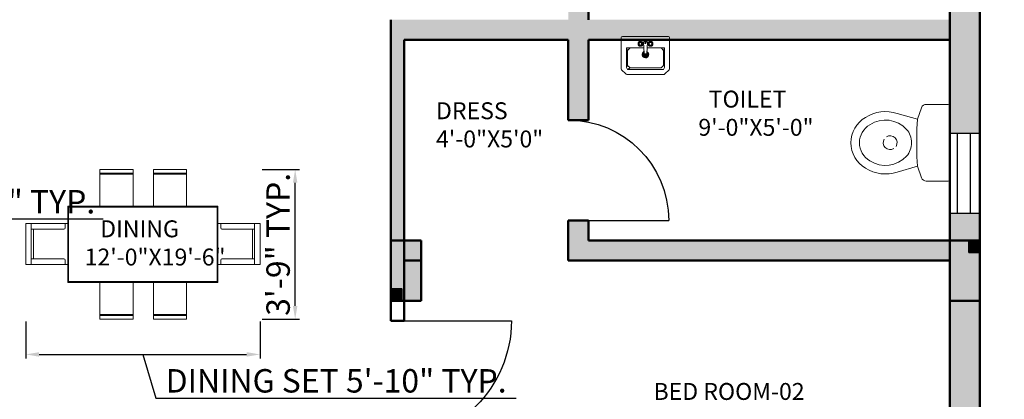
# Model space of a CAD drawing. Units: inches. Extents: x -7 to 1228, y -146 to 1091.
# Tile 23 of 88: x 269 to 563, y 194 to 307. Entities that reach past the tile are written whole.
import ezdxf

# ---------------------------------------------------------------- set-up
doc = ezdxf.new("R2010")
doc.units = ezdxf.units.IN
for name, color, linetype, lineweight in [('A-ANNO-DIMS', 2, 'Continuous', 18), ('A-AREA-IDEN', 7, 'Continuous', 18), ('A-COLS', 6, 'Continuous', 35), ('A-DOOR', 4, 'Continuous', 25), ('A-FLOR-FIXT', 8, 'Continuous', 18), ('A-FURN', 8, 'Continuous', 18), ('A-GLAZ', 175, 'Continuous', 25), ('A-WALL', 7, 'Continuous', 50), ('A-WALL-PATT', 251, 'Continuous', 13)]:
    doc.layers.add(name, color=color, linetype=linetype, lineweight=lineweight)
doc.styles.get("Standard").update_dxf_attribs({"font": 'arial.ttf'})
doc.dimstyles.new('ISO-25', dxfattribs={"dimtxt": 7, "dimasz": 4, "dimexe": 1.25, "dimexo": 0.625, "dimtad": 1, "dimdec": 1, "dimlunit": 3, "dimtxsty": 'Standard', "dimcen": 2.5, "dimadec": 0, "dimazin": 0, "dimtfac": 1, "dimtdec": 1, "dimtmove": 1, "dimatfit": 3, "dimfxl": 1, "dimarcsym": 0})

# ---------------------------------------------------------------- blocks, each defined once
blk = doc.blocks.new('A$C7B5C7CD4')
at = {"ltscale": 20}
for p, q in [((0.243, 0.625), (0.011, 0.625)), ((0.243, 0.625), (0.475, 0.625)), ((0, 0.614), (0, 0.4765)), ((0.486, 0.614), (0.486, 0.4765)), ((0.0212, 0.4467), (0.0946, 0.4214)), ((0.4648, 0.4467), (0.3914, 0.4214)), ((0.0946, 0.4214), (0.0576, 0.293)), ((0.0946, 0.4214), (0.1544, 0.4173)), ((0.3316, 0.4173), (0.1544, 0.4173)), ((0.3914, 0.4214), (0.3316, 0.4173)), ((0.3914, 0.4214), (0.4284, 0.293))]:
    blk.add_line(p, q, dxfattribs=at)
for centre, radius, start, end in [((0.011, 0.614), 0.011, 90, 180), ((0.475, 0.614), 0.011, 0, 90), ((0.0315, 0.4765), 0.0315, 180, 251), ((0.4545, 0.4765), 0.0315, 289, 0), ((0.24, 0.2602), 0.123, 88.61575, 131.74141), ((0.246, 0.2602), 0.123, 48.25859, 91.38425), ((0.2796, 0.219), 0.18, 132.42075, 213.28898), ((0.2064, 0.219), 0.18, 326.71102, 47.57925), ((0.2796, 0.219), 0.234, 161.58462, 212.87535), ((0.2064, 0.219), 0.234, 327.12465, 18.41538), ((0.243, 0.185), 0.185, 210.1745, 270), ((0.243, 0.185), 0.131, 209.62919, 270), ((0.243, 0.185), 0.131, 270, 330.37081), ((0.243, 0.185), 0.185, 270, 329.8255)]:
    blk.add_arc(centre, radius, start, end, dxfattribs=at)
for start, end in [(58.17854, 211.82146), (238.17854, 31.82146)]:
    blk.add_arc((0.2426, 0.2481), 0.0439, start, end)
blk = doc.blocks.new('A$C317A697B')
for p, q in [((-116, 441), (-514, 441)), ((-514, 441), (-514, 0)), ((-116, 398), (-514, 398)), ((-116, 385), (-514, 385)), ((-116, 0), (-116, 441)), ((523, 441), (125, 441)), ((125, 441), (125, 0)), ((523, 398), (125, 398)), ((523, 385), (125, 385)), ((523, 0), (523, 441)), ((-899, -912), (-899, 0)), ((-899, 0), (899, 0)), ((899, 0), (899, -912)), ((-889, -902), (-889, -10)), ((-889, -10), (889, -10)), ((889, -10), (889, -902)), ((-899, -205), (-1402, -205)), ((-1402, -205), (-1402, -699)), ((-1336, -205), (-1336, -699)), ((-932, -205), (-932, -259)), ((899, -205), (1402, -205)), ((932, -205), (932, -259)), ((1336, -205), (1336, -699)), ((1402, -205), (1402, -699)), ((-946, -274), (-1336, -274)), ((-1311, -274), (-1311, -630)), ((946, -274), (1336, -274)), ((1311, -274), (1311, -630)), ((-1402, -699), (-899, -699)), ((-946, -630), (-1336, -630)), ((-932, -699), (-932, -645)), ((1402, -699), (899, -699)), ((932, -699), (932, -645)), ((946, -630), (1336, -630)), ((899, -912), (-899, -912)), ((889, -902), (-889, -902)), ((-514, -1353), (-514, -912)), ((-116, -912), (-116, -1353)), ((125, -1353), (125, -912)), ((523, -912), (523, -1353)), ((-116, -1297), (-514, -1297)), ((-116, -1309), (-514, -1309)), ((-116, -1353), (-514, -1353)), ((523, -1297), (125, -1297)), ((523, -1309), (125, -1309)), ((523, -1353), (125, -1353))]:
    blk.add_line(p, q)
for centre, start, end in [((-946, -259), 270, 0), ((946, -259), 180, 270), ((-946, -645), 0, 90), ((946, -645), 90, 180)]:
    blk.add_arc(centre, 14.7, start, end)
blk = doc.blocks.new('A$C4CB854FF')
for p, q in [((0, 0.3675), (0, 0.0552)), ((0.4725, 0.38), (0.0125, 0.38)), ((0.1677, 0.2932), (0.1677, 0.318)), ((0.1745, 0.2919), (0.1745, 0.3194)), ((0.1773, 0.3221), (0.2048, 0.3221)), ((0.1787, 0.329), (0.2034, 0.329)), ((0.2075, 0.3194), (0.2075, 0.2919)), ((0.2144, 0.318), (0.2144, 0.2932)), ((0.2279, 0.2104), (0.2213, 0.3235)), ((0.2337, 0.329), (0.2502, 0.329)), ((0.2625, 0.3235), (0.256, 0.2104)), ((0.2694, 0.318), (0.2694, 0.2932)), ((0.2763, 0.3194), (0.2763, 0.2919)), ((0.3065, 0.3221), (0.279, 0.3221)), ((0.3052, 0.329), (0.2804, 0.329)), ((0.3093, 0.2919), (0.3093, 0.3194)), ((0.3162, 0.2932), (0.3162, 0.318)), ((0.485, 0.0552), (0.485, 0.3675)), ((0.05, 0.265), (0.2247, 0.265)), ((0.06, 0.24), (0.05, 0.265)), ((0.05, 0.07), (0.05, 0.265)), ((0.085, 0.265), (0.06, 0.24)), ((0.06, 0.24), (0.06, 0.09)), ((0.2048, 0.2891), (0.1773, 0.2891)), ((0.2034, 0.2822), (0.1787, 0.2822)), ((0.2152, 0.1984), (0.2694, 0.1984)), ((0.2297, 0.2066), (0.2165, 0.2066)), ((0.2272, 0.2149), (0.2208, 0.2149)), ((0.2505, 0.2052), (0.2334, 0.2052)), ((0.2681, 0.2066), (0.2541, 0.2066)), ((0.2638, 0.2149), (0.2566, 0.2149)), ((0.2591, 0.265), (0.43, 0.265)), ((0.279, 0.2891), (0.3065, 0.2891)), ((0.2804, 0.2822), (0.3052, 0.2822)), ((0.395, 0.265), (0.42, 0.24)), ((0.42, 0.24), (0.43, 0.265)), ((0.42, 0.24), (0.42, 0.09)), ((0.43, 0.07), (0.43, 0.265)), ((0.2681, 0.1901), (0.2165, 0.1901)), ((0.2638, 0.1819), (0.2208, 0.1819)), ((0.2533, 0.1736), (0.2313, 0.1736)), ((0.0037, 0.0463), (0.0463, 0.0037)), ((0.05, 0.07), (0.06, 0.05)), ((0.06, 0.09), (0.085, 0.065)), ((0.42, 0.05), (0.06, 0.05)), ((0.085, 0.065), (0.395, 0.065)), ((0.42, 0.09), (0.395, 0.065)), ((0.395, 0.065), (0.42, 0.05)), ((0.42, 0.09), (0.43, 0.07)), ((0.43, 0.07), (0.42, 0.05)), ((0.4387, 0.0037), (0.4813, 0.0463)), ((0.0552, 0), (0.4298, 0))]:
    blk.add_line(p, q)
for centre, radius in [((0.191, 0.3056), 0.0165), ((0.191, 0.3056), 0.0127), ((0.2419, 0.3152), 0.00688), ((0.2419, 0.3152), 0.00344), ((0.2928, 0.3056), 0.0165), ((0.2928, 0.3056), 0.0127)]:
    blk.add_circle(centre, radius)
for centre, radius, start, end in [((0.0125, 0.3675), 0.0125, 90, 180), ((0.1787, 0.318), 0.011, 90, 180), ((0.1773, 0.3194), 0.00275, 90, 180), ((0.2034, 0.318), 0.011, 0, 90), ((0.2048, 0.3194), 0.00275, 360, 90), ((0.2329, 0.314), 0.015, 87.19754, 140.72744), ((0.2509, 0.314), 0.015, 39.27256, 92.80246), ((0.2804, 0.318), 0.011, 90, 180), ((0.279, 0.3194), 0.00275, 90, 180), ((0.3052, 0.318), 0.011, 0, 90), ((0.3065, 0.3194), 0.00275, 360, 90), ((0.4725, 0.3675), 0.0125, 0, 90), ((0.1787, 0.2932), 0.011, 180, 270), ((0.1773, 0.2919), 0.00275, 180, 270), ((0.2034, 0.2932), 0.011, 270, 0), ((0.2048, 0.2919), 0.00275, 270, 0), ((0.2423, 0.1984), 0.033, 118.68833, 62.86857), ((0.2423, 0.1984), 0.0271, 124.77581, 57.22467), ((0.2334, 0.2107), 0.0055, 183.3274, 270), ((0.2505, 0.2107), 0.0055, 270, 356.6726), ((0.2804, 0.2932), 0.011, 180, 270), ((0.279, 0.2919), 0.00275, 180, 270), ((0.3052, 0.2932), 0.011, 270, 360), ((0.3065, 0.2919), 0.00275, 270, 0), ((0.0125, 0.0552), 0.0125, 180, 225), ((0.0552, 0.0125), 0.0125, 225, 270), ((0.4298, 0.0125), 0.0125, 270, 315), ((0.4725, 0.0552), 0.0125, 315, 0)]:
    blk.add_arc(centre, radius, start, end)
blk = doc.blocks.new('WIN-24')
for p, q in [((0, 0), (0, 24)), ((0, 24), (9, 24)), ((2.34, 0), (2.34, 24)), ((2.34, 24), (6.14, 24)), ((6.14, 24), (6.14, 0)), ((9, 24), (9, 0)), ((9, 0), (0, 0))]:
    blk.add_line(p, q)
blk = doc.blocks.new('DOOR-750')
blk.add_line((30, 30), (30, 0))
blk.add_arc((30, 30), 30, 180, 270)
blk = doc.blocks.new('DOOR-900')
blk.add_line((36, 0), (36, 36))
blk.add_arc((36, 0), 36, 90, 180)
blk = doc.blocks.new('*D32')
at = {"layer": 'A-ANNO-DIMS', "color": 0, "lineweight": -2, "transparency": 16777216}
for p, q in [((159.65, 262.03), (159.65, 259.24)), ((174.13, 262.03), (174.13, 259.24)), ((170.13, 260.49), (163.65, 260.49)), ((166.89, 260.49), (170.8, 247.44)), ((170.8, 247.44), (294.04, 247.44))]:
    blk.add_line(p, q, dxfattribs=at)
at = {"layer": 'A-ANNO-DIMS', "color": 0, "transparency": 16777216}
for points in [[(163.65, 261.15), (163.65, 259.82), (159.65, 260.49)], [(170.13, 261.15), (170.13, 259.82), (174.13, 260.49)]]:
    blk.add_solid(points, dxfattribs=at)
at = {"layer": 'Defpoints', "color": 0, "transparency": 16777216}
for p in [(159.65, 262.66), (174.13, 262.66), (159.65, 260.49)]:
    blk.add_point(p, dxfattribs=at)
at = {"layer": 'A-ANNO-DIMS', "color": 0, "transparency": 16777216, "insert": (232.42, 251.68), "char_height": 7, "attachment_point": 5}
blk.add_mtext('SINK / BASIN 1\'-2 1/2" TYP.', dxfattribs=at)
blk = doc.blocks.new('*D36')
at = {"layer": 'A-ANNO-DIMS', "color": 0, "lineweight": -2, "transparency": 16777216}
for p, q in [((270.86, 216.83), (270.86, 205.7)), ((340.87, 216.83), (340.87, 205.7)), ((274.86, 206.95), (336.87, 206.95)), ((305.87, 206.95), (309.78, 193.91)), ((309.78, 193.91), (417.47, 193.91))]:
    blk.add_line(p, q, dxfattribs=at)
at = {"layer": 'A-ANNO-DIMS', "color": 0, "transparency": 16777216}
for points in [[(274.86, 207.62), (274.86, 206.28), (270.86, 206.95)], [(336.87, 207.62), (336.87, 206.28), (340.87, 206.95)]]:
    blk.add_solid(points, dxfattribs=at)
at = {"layer": 'Defpoints', "color": 0, "transparency": 16777216}
for p in [(270.86, 217.45), (340.87, 217.45), (340.87, 206.95)]:
    blk.add_point(p, dxfattribs=at)
at = {"layer": 'A-ANNO-DIMS', "color": 0, "transparency": 16777216, "insert": (363.62, 198.15), "char_height": 7, "attachment_point": 5}
blk.add_mtext('DINING SET 5\'-10" TYP.', dxfattribs=at)
blk = doc.blocks.new('*D37')
at = {"layer": 'A-ANNO-DIMS', "color": 0, "lineweight": -2, "transparency": 16777216}
for p, q in [((341.5, 262.25), (352.63, 262.25)), ((351.38, 221.45), (351.38, 258.25)), ((341.5, 217.45), (352.63, 217.45))]:
    blk.add_line(p, q, dxfattribs=at)
at = {"layer": 'A-ANNO-DIMS', "color": 0, "transparency": 16777216}
for points in [[(350.71, 258.25), (352.04, 258.25), (351.38, 262.25)], [(350.71, 221.45), (352.04, 221.45), (351.38, 217.45)]]:
    blk.add_solid(points, dxfattribs=at)
at = {"layer": 'Defpoints', "color": 0, "transparency": 16777216}
for p in [(340.87, 262.25), (351.38, 262.25), (340.87, 217.45)]:
    blk.add_point(p, dxfattribs=at)
at = {"layer": 'A-ANNO-DIMS', "color": 0, "transparency": 16777216, "insert": (347.18, 239.85), "char_height": 7, "attachment_point": 5, "rotation": 90}
blk.add_mtext('3\'-9" TYP.', dxfattribs=at)

msp = doc.modelspace()

# ---------------------------------------------------------------- hatches: boundary and pattern name
at = {"layer": 'A-COLS'}
h = msp.add_hatch(color=256, dxfattribs=at)
h.dxf.hatch_style = 1
h.paths.add_polyline_path([(380, 226.55), (383.29, 226.55), (383.29, 223), (389, 223), (389, 241), (380, 241)])
h = msp.add_hatch(color=256, dxfattribs=at)
h.dxf.hatch_style = 1
h.paths.add_polyline_path([(556, 237.45), (552.71, 237.45), (552.71, 241), (547, 241), (547, 223), (556, 223)])
h = msp.add_hatch(color=256, dxfattribs=at)
h.dxf.hatch_style = 1
h.paths.add_polyline_path([(556, 237.45), (556, 241), (552.71, 241), (552.71, 237.45)])
h = msp.add_hatch(color=256, dxfattribs=at)
h.dxf.hatch_style = 1
h.paths.add_polyline_path([(380, 226.55), (380, 223), (383.29, 223), (383.29, 226.55)])
at = {"layer": 'A-WALL-PATT'}
h = msp.add_hatch(color=256, dxfattribs=at)
h.dxf.hatch_style = 1
h.paths.add_polyline_path([(69, 568), (60, 568), (60, 493), (63.29, 493), (69, 493)])
h.paths.add_polyline_path([(69, 662.41), (60, 662.41), (60, 586), (69, 586)], flags=17)
h.paths.add_polyline_path([(69, 723), (184, 723), (184, 734), (179, 734), (179, 728), (69, 728), (69, 741.62), (60, 741.62), (60, 698.41), (69, 698.41)], flags=17)
h.paths.add_polyline_path([(69, 782), (231, 782), (231, 728), (231, 723), (231, 586), (236, 586), (236, 787), (69, 787), (69, 800.13), (60, 800.13), (60, 765.62), (69, 765.62)])
h.paths.add_polyline_path([(184, 842), (189, 842), (189, 848), (173, 848), (173, 842), (179, 842), (179, 787), (184, 787)])
h.paths.add_polyline_path([(118.22, 69), (69, 69), (69, 60), (118.22, 60)])
h.paths.add_polyline_path([(227, 69), (154.22, 69), (154.22, 60), (227, 60)])
h.paths.add_polyline_path([(236, 60), (232.71, 60), (227, 60), (227, 36), (236, 36)])
h.paths.add_polyline_path([(389, 60), (380, 60), (380, 36), (389, 36)])
h.paths.add_polyline_path([(384, 181), (380, 181), (380, 115), (380, 78), (384, 78)])
h.paths.add_polyline_path([(380, 115), (334.55, 115), (334.55, 109), (380, 109)])
h.paths.add_polyline_path([(274.55, 115), (236, 115), (236, 201), (232.71, 201), (231, 201), (231, 78), (236, 78), (236, 109), (274.55, 109)])
h.paths.add_polyline_path([(69, 123), (60, 123), (60, 78), (69, 78)])
h.paths.add_polyline_path([(69, 201), (60, 201), (60, 159), (69, 159)])
h.paths.add_polyline_path([(143, 219), (69, 219), (69, 213), (143, 213)], flags=17)
h.paths.add_polyline_path([(189, 219), (184, 219), (184, 274), (231, 274), (231, 219), (236, 219), (236, 279), (184, 279), (184, 297), (179, 297), (179, 279), (69, 279), (69, 290.91), (60, 290.91), (60, 262.18), (69, 262.18), (69, 274), (179, 274), (179, 219), (173, 219), (173, 213), (189, 213)])
h.paths.add_polyline_path([(69, 238.18), (60, 238.18), (60, 219), (69, 219)], flags=17)
h.paths.add_polyline_path([(69, 333), (60, 333), (60, 314.91), (69, 314.91), (69, 316.96)])
h.paths.add_polyline_path([(190, 338), (184, 338), (69, 338), (69, 333), (179, 333), (179, 327), (184, 327), (184, 333.02), (190, 333.05)])
h.paths.add_polyline_path([(69, 386.81), (60, 386.81), (60, 351), (69, 351)])
h.paths.add_polyline_path([(69, 475), (60, 475), (60, 422.81), (69, 422.81)])
h.paths.add_polyline_path([(236, 475), (231, 475), (231, 351.24), (236, 351.24)])
h.paths.add_polyline_path([(384, 475), (380, 475), (380, 362), (384, 362)])
h.paths.add_polyline_path([(547, 307), (439, 307), (439, 356), (445, 356), (445, 362), (433, 362), (433, 307), (380, 307), (380, 244), (380, 241), (384, 241), (384, 301), (433, 301), (433, 277), (439, 277), (439, 301), (547, 301)])
h.paths.add_polyline_path([(547, 241), (439, 241), (439, 247), (433, 247), (433, 235), (547, 235)])
h.paths.add_polyline_path([(450, 69), (440.29, 69), (424.89, 69), (389, 69), (389, 60), (450, 60)])
h.paths.add_polyline_path([(547, 69), (486, 69), (486, 60), (547, 60)])
h.paths.add_polyline_path([(556, 148.27), (547, 148.27), (547, 78), (556, 78)])
h.paths.add_polyline_path([(556, 223), (547, 223), (547, 195), (547, 184.27), (556, 184.27)])
h.paths.add_polyline_path([(556, 311.19), (547, 311.19), (547, 273.08), (556, 273.08)])
h.paths.add_polyline_path([(556, 344), (552.71, 344), (547, 344), (547, 335.19), (556, 335.19)])
h.paths.add_polyline_path([(556, 249.08), (547, 249.08), (547, 241), (556, 241)])
h.paths.add_polyline_path([(547, 362), (475, 362), (475, 356), (547, 356)], flags=0)
h.paths.add_polyline_path([(556, 399.62), (547, 399.62), (547, 362), (556, 362)])
h.paths.add_polyline_path([(556, 475), (547, 475), (547, 435.62), (556, 435.62)])
h.paths.add_polyline_path([(547, 493), (389, 493), (389, 487), (547, 487)])
h.paths.add_polyline_path([(380, 493), (278, 493), (278, 487), (380, 487)])
h.paths.add_polyline_path([(227, 493), (69, 493), (69, 487), (227, 487)])
h.paths.add_polyline_path([(643, 122.44), (634, 122.44), (634, 78), (643, 78)])
h.paths.add_polyline_path([(702.5, 69), (692.79, 69), (677.39, 69), (643, 69), (643, 60), (702.5, 60)])
h.paths.add_polyline_path([(798, 69), (738.5, 69), (738.5, 60), (798, 60)])
h.paths.add_polyline_path([(807, 60), (803.71, 60), (798, 60), (798, 36), (807, 36)])
h.paths.add_polyline_path([(807, 109), (846.75, 109), (846.75, 115), (807, 115), (807, 159), (802, 159), (802, 78), (807, 78)])
h.paths.add_polyline_path([(807, 201), (802, 201), (802, 195), (807, 195)])
h.paths.add_polyline_path([(643, 201), (634, 201), (634, 158.44), (643, 158.44)])
h.paths.add_polyline_path([(756, 225), (751, 225), (751, 219), (643, 219), (643, 213), (756, 213)])
h.paths.add_polyline_path([(643, 240.85), (634, 240.85), (634, 219), (643, 219)])
h.paths.add_polyline_path([(643, 274), (643, 288.63), (634, 288.63), (634, 264.85), (643, 264.85)])
h.paths.add_polyline_path([(802, 279), (756, 279), (756, 297), (751, 297), (751, 279), (643, 279), (643, 274), (751, 274), (751, 255), (756, 255), (756, 274), (802, 274)])
h.paths.add_polyline_path([(807, 333), (803.71, 333), (802, 333), (802, 279), (802, 274), (802, 219), (807, 219)])
h.paths.add_polyline_path([(956, 182), (951, 182), (951, 115), (906.75, 115), (906.75, 109), (951, 109), (951, 78), (956, 78)])
h.paths.add_polyline_path([(960, 60), (951, 60), (951, 36), (960, 36)])
h.paths.add_polyline_path([(1021, 69), (1005.78, 69), (960, 69), (960, 60), (1021, 60)])
h.paths.add_polyline_path([(956, 224), (951, 224), (951, 218), (956, 218)])
h.paths.add_polyline_path([(956, 302), (1004, 302), (1004, 278), (1010, 278), (1010, 302), (1118, 302), (1118, 290.81), (1127, 290.81), (1127, 326.97), (1118, 326.97), (1118, 320.97), (1118, 307), (1010, 307), (1010, 356), (1016, 356), (1016, 362), (1004, 362), (1004, 307), (951, 307), (951, 244), (951, 242), (954.29, 242), (956, 242)])
h.paths.add_polyline_path([(643, 333), (634, 333), (634, 312.63), (643, 312.63), (643, 316.96)])
h.paths.add_polyline_path([(756, 338), (643, 338), (643, 333), (751, 333), (751, 327), (756, 327)])
h.paths.add_polyline_path([(643, 388), (634, 388), (634, 351), (643, 351)])
h.paths.add_polyline_path([(807, 357), (802, 357), (802, 351), (807, 351)])
h.paths.add_polyline_path([(807, 475), (802, 475), (802, 393), (807, 393)])
h.paths.add_polyline_path([(643, 475), (634, 475), (634, 424), (643, 424)])
h.paths.add_polyline_path([(798, 493), (643, 493), (643, 487), (798, 487)])
h.paths.add_polyline_path([(634, 493), (556, 493), (556, 487), (634, 487)])
h.paths.add_polyline_path([(813, 493), (807, 493), (807, 487), (813, 487)])
h.paths.add_polyline_path([(951, 493), (849, 493), (849, 487), (951, 487)])
h.paths.add_polyline_path([(956, 484), (951, 484), (951, 374), (956, 374)])
h.paths.add_polyline_path([(1109, 493), (969, 493), (969, 487), (1109, 487)])
h.paths.add_polyline_path([(1127, 484), (1118, 484), (1118, 450.64), (1127, 450.64)])
h.paths.add_polyline_path([(1127, 414.64), (1118, 414.64), (1118, 365), (1127, 365)])
h.paths.add_polyline_path([(1109, 362), (1046, 362), (1046, 356), (1109, 356)], flags=17)
h.paths.add_polyline_path([(1127, 356), (1123.45, 356), (1118, 356), (1118, 350.97), (1127, 350.97)], flags=0)
h.paths.add_polyline_path([(1127, 266.81), (1118, 266.81), (1118, 262.36), (1118, 242), (1127, 242)], flags=17)
h.paths.add_polyline_path([(1118, 242), (1010, 242), (1010, 248), (1004, 248), (1004, 237), (1118, 237)])
h.paths.add_polyline_path([(1127, 224), (1118, 224), (1118, 170), (1127, 170)])
h.paths.add_polyline_path([(1127, 134), (1118, 134), (1118, 78), (1127, 78)])
h.paths.add_polyline_path([(1118, 69), (1057, 69), (1057, 60), (1118, 60)])
h.paths.add_polyline_path([(227, 571.55), (227, 574), (69, 574), (69, 568), (227, 568)])
h.paths.add_polyline_path([(380, 571.55), (380, 574), (278, 574), (278, 568), (380, 568)])
h.paths.add_polyline_path([(242, 574), (236, 574), (236, 568), (242, 568)])
h.paths.add_polyline_path([(547, 571.55), (547, 574), (389, 574), (389, 568), (547, 568)])
h.paths.add_polyline_path([(384, 733), (380, 733), (380, 586), (384, 586)])
h.paths.add_polyline_path([(556, 646), (634, 646), (634, 655), (547, 655), (547, 586), (556, 586)])
h.paths.add_polyline_path([(634, 574), (556, 574), (556, 568), (634, 568)])
h.paths.add_polyline_path([(643, 655), (634, 655), (634, 586), (643, 586)])
h.paths.add_polyline_path([(798, 574), (643, 574), (643, 568), (798, 568)])
h.paths.add_polyline_path([(643, 663.85), (634, 663.85), (634, 655), (643, 655)])
h.paths.add_polyline_path([(556, 676.97), (547, 676.97), (547, 655), (556, 655)])
h.paths.add_polyline_path([(556, 733), (547, 733), (547, 712.97), (556, 712.97)])
h.paths.add_polyline_path([(643, 710), (634, 710), (634, 699.85), (643, 699.85)])
h.paths.add_polyline_path([(807, 668), (802, 668), (802, 586), (807, 586)])
h.paths.add_polyline_path([(951, 574), (849, 574), (849, 568), (951, 568)])
h.paths.add_polyline_path([(956, 691), (951, 691), (951, 577), (956, 577)])
h.paths.add_polyline_path([(1109, 574), (969, 574), (969, 568), (1109, 568)])
h.paths.add_polyline_path([(1127, 643.4), (1118, 643.4), (1118, 577), (1127, 577)])
h.paths.add_polyline_path([(1127, 568), (1123.45, 568), (1118, 568), (1118, 493), (1127, 493)])
h.paths.add_polyline_path([(1127, 733), (1118, 733), (1118, 679.4), (1127, 679.4)])
h.paths.add_polyline_path([(1127, 777.35), (1118, 777.35), (1118, 770.04), (1118, 751), (1127, 751)], flags=17)
h.paths.add_polyline_path([(1118, 751), (1010, 751), (1010, 757), (1004, 757), (1004, 745), (1118, 745)])
h.paths.add_polyline_path([(956, 811), (1004, 811), (1004, 787), (1010, 787), (1010, 811), (1017.87, 811), (1017.87, 811.63, -0.414214), (1018.25, 812), (1031.98, 812, -0.414214), (1032.35, 811.63), (1032.35, 811), (1118, 811), (1118, 801.35), (1127, 801.35), (1127, 834.69), (1118, 834.69), (1118, 830.24), (1118, 817), (1010, 817), (1010, 866), (1016, 866), (1016, 872), (1004, 872), (1004, 817), (956, 817), (956, 866), (951, 866), (951, 751), (954.29, 751), (956, 751)])
h.paths.add_polyline_path([(1118, 872), (1046, 872), (1046, 866), (1118, 866)], flags=17)
h.paths.add_polyline_path([(1127, 924.71), (1118, 924.71), (1118, 884), (1127, 884)])
h.paths.add_polyline_path([(1127, 866), (1123.71, 866), (1118, 866), (1118, 858.69), (1127, 858.69)], flags=17)
h.paths.add_polyline_path([(956, 983), (951, 983), (951, 952), (807, 952), (807, 983), (802, 983), (802, 902), (807, 902), (807, 946), (951, 946), (951, 884), (956, 884)])
h.paths.add_polyline_path([(807, 842), (802, 842), (802, 787), (756, 787), (756, 806), (751, 806), (751, 787), (643, 787), (643, 782), (751, 782), (751, 764), (756, 764), (756, 782), (802, 782), (802, 728), (807, 728)])
h.paths.add_polyline_path([(756, 848), (643, 848), (643, 842), (751, 842), (751, 836), (756, 836)])
h.paths.add_polyline_path([(756, 734), (751, 734), (751, 728), (643, 728), (643, 723), (756, 723)])
h.paths.add_polyline_path([(643, 749.79), (634, 749.79), (634, 728), (637.29, 728), (643, 728)])
h.paths.add_polyline_path([(643, 805.41), (634, 805.41), (634, 773.79), (643, 773.79)])
h.paths.add_polyline_path([(643, 896.66), (634, 896.66), (634, 860), (637.29, 860), (643, 860)])
h.paths.add_polyline_path([(643, 842), (634, 842), (634, 829.41), (643, 829.41)])
h.paths.add_polyline_path([(643, 983), (634, 983), (634, 932.66), (643, 932.66)])
h.paths.add_polyline_path([(1127, 983), (1118, 983), (1118, 960.71), (1127, 960.71)])
h.paths.add_polyline_path([(1118, 1001), (1077.53, 1001), (1077.53, 992), (1118, 992)])
h.paths.add_polyline_path([(1041.53, 1001), (960, 1001), (960, 992), (1041.53, 992)])
h.paths.add_polyline_path([(960, 1025), (951, 1025), (951, 1001), (954.29, 1001), (960, 1001)])
h.paths.add_polyline_path([(807, 1025), (798, 1025), (798, 1001), (807, 1001)])
h.paths.add_polyline_path([(798, 1001), (738.5, 1001), (738.5, 992), (798, 992)])
h.paths.add_polyline_path([(702.5, 1001), (643, 1001), (643, 992), (702.5, 992)])
h.paths.add_polyline_path([(547, 1001), (499.11, 1001), (499.11, 992), (547, 992)])
h.paths.add_polyline_path([(463.11, 1001), (389, 1001), (389, 992), (463.11, 992)])
h.paths.add_polyline_path([(389, 1025), (380, 1025), (380, 1022), (380, 1001), (383.29, 1001), (389, 1001)])
h.paths.add_polyline_path([(236, 1025), (227, 1025), (227, 1001), (236, 1001)])
h.paths.add_polyline_path([(236, 983), (231, 983), (231, 860), (236, 860)])
h.paths.add_polyline_path([(274.55, 952), (236, 952), (236, 946), (274.55, 946)])
h.paths.add_polyline_path([(380, 952), (334.55, 952), (334.55, 946), (380, 946)])
h.paths.add_polyline_path([(384, 983), (380, 983), (380, 884), (383.29, 884), (384, 884)])
h.paths.add_polyline_path([(227, 1001), (155.01, 1001), (155.01, 992), (162.87, 992), (227, 992)])
h.paths.add_polyline_path([(119.01, 1001), (69, 1001), (69, 992), (119.01, 992)])
h.paths.add_polyline_path([(69, 983), (60, 983), (60, 922.99), (69, 922.99)])
h.paths.add_polyline_path([(69, 886.99), (60, 886.99), (60, 860), (63.29, 860), (69, 860)])
h.paths.add_polyline_path([(143, 848), (69, 848), (69, 842), (143, 842)])

# ---------------------------------------------------------------- linework, layer by layer
at = {"layer": 'A-COLS'}
for points in [[(556, 241), (552.71, 241), (552.71, 237.45), (556, 237.45)], [(380, 223), (383.29, 223), (383.29, 226.55), (380, 226.55)]]:
    msp.add_lwpolyline(points, close=True, dxfattribs=at)
at = {"layer": 'A-WALL'}
for p, q in [((547, 493), (547, 60)), ((556, 493), (556, 60)), ((556, 60), (556, 406)), ((439, 307), (439, 356)), ((547, 250), (547, 310)), ((380, 244), (380, 307)), ((380, 307), (380, 217)), ((384, 250), (384, 301)), ((433, 301), (384, 301)), ((384, 301), (384, 217)), ((433, 277), (433, 301)), ((547, 301), (439, 301)), ((439, 277), (439, 301)), ((439, 277), (433, 277)), ((433, 235), (433, 247)), ((439, 247), (433, 247)), ((439, 241), (439, 247)), ((547, 195), (547, 244)), ((389, 241), (380, 241)), ((380, 241), (380, 223)), ((389, 241), (384, 241)), ((389, 223), (389, 241)), ((389, 241), (389, 235)), ((547, 241), (439, 241)), ((556, 241), (547, 241)), ((547, 241), (547, 223)), ((556, 223), (556, 241)), ((389, 235), (384, 235)), ((547, 235), (433, 235)), ((380, 223), (389, 223)), ((384, 223), (380, 223)), ((547, 223), (556, 223)), ((384, 217), (380, 217))]:
    msp.add_line(p, q, dxfattribs=at)

# ---------------------------------------------------------------- block references
at = {"layer": 'A-DOOR', "extrusion": (0, 0, -1), "zscale": -1}
for name, p, rotation in [('DOOR-750', (-463, 277), 269.9999999999998), ('DOOR-900', (-380, 181), 89.99999999999969)]:
    msp.add_blockref(name, p, dxfattribs=dict(at, rotation=rotation))
at = {"layer": 'A-FLOR-FIXT', "xscale": 47.26153857112405, "yscale": 47.26153857112405, "zscale": 47.26153857112405, "rotation": 270}
msp.add_blockref('A$C7B5C7CD4', (517.46, 281.7), dxfattribs=at)
at = {"layer": 'A-FURN'}
for name, p, xscale, yscale, zscale in [('A$C4CB854FF', (463.28, 290.66), -29.84864686937646, 29.84864686937646, 29.84864686937646), ('A$C317A697B', (305.87, 251.23), 0.024965713951469, 0.024965713951469, 0.024965713951469)]:
    msp.add_blockref(name, p, dxfattribs=dict(at, xscale=xscale, yscale=yscale, zscale=zscale))
at = {"layer": 'A-GLAZ'}
msp.add_blockref('WIN-24', (547, 249.07), dxfattribs=at)

# ---------------------------------------------------------------- texts
at = {"layer": 'A-AREA-IDEN', "attachment_point": 1}
for s, insert, char_height in [('  TOILET\\P9\'-0"X5\'-0"', (471.87, 285.79), 5.0568), ('DRESS\\P4\'-0"X5\'0"', (393.47, 282.31), 5.057), ('   DINING\\P12\'-0"X19\'-6"', (288.47, 247.02), 5.0568), ('BED ROOM-02\\P13\'-6"X12\'-0"', (458.47, 198.41), 5.0568)]:
    msp.add_mtext_dynamic_manual_height_columns(s, width=137.2821, gutter_width=25.28, heights=[0], dxfattribs=dict(at, insert=insert, char_height=char_height))

# ---------------------------------------------------------------- dimensions: what is measured, and where the dimension line sits
at = {"layer": 'A-ANNO-DIMS'}
for base, p1, p2, angle, text, picture, middle in [((159.65, 260.49), (174.13, 262.66), (159.65, 262.66), 180, 'SINK / BASIN <> TYP.', '*D32', (171.43, 251.68)), ((351.38, 262.25), (340.87, 217.45), (340.87, 262.25), 90, '<> TYP.', '*D37', (347.18, 239.85))]:
    dim = msp.add_linear_dim(base=base, p1=p1, p2=p2, angle=angle, text=text, dimstyle='ISO-25', override={"dimdec": 1, "dimlfac": 1, "dimrnd": 0, "dimzin": 1, "dimdsep": 46, "dimlunit": 4, "dimfrac": 2}, dxfattribs=at)
    dim.commit()
    dim.dimension.update_dxf_attribs({"geometry": picture, "text_midpoint": middle})
dim = msp.add_linear_dim(base=(340.87, 206.95), p1=(270.86, 217.45), p2=(340.87, 217.45), text='DINING SET <> TYP.', dimstyle='ISO-25', override={"dimdec": 1, "dimlfac": 1, "dimrnd": 0, "dimzin": 1, "dimdsep": 46, "dimlunit": 4, "dimfrac": 2}, dxfattribs=at)
dim.commit()
dim.dimension.update_dxf_attribs({"geometry": '*D36', "text_midpoint": (310.4, 198.15)})

doc.saveas('drawing.dxf')
